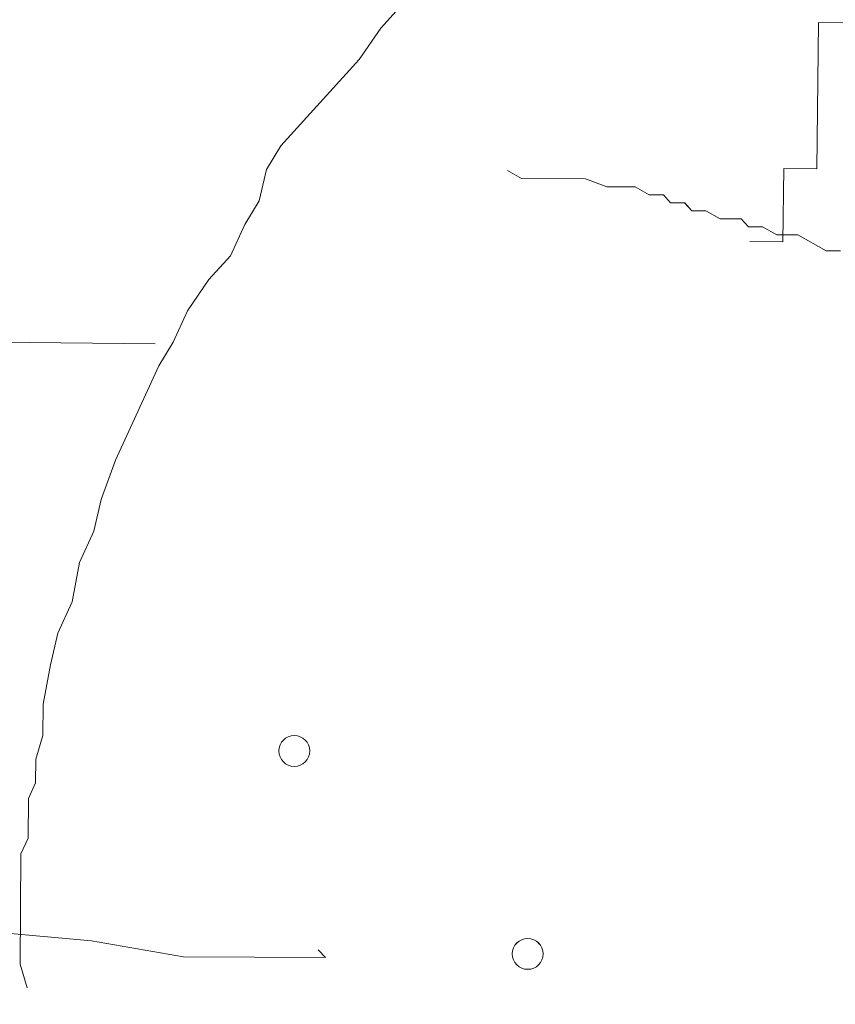
# Model space of a CAD drawing. Units: inches. Extents: x -466983 to 1020, y 324 to 318697.
# Tile 58 of 97: x 640.764 to 643.839, y 938.98 to 942.694. Entities that reach past the tile are written whole.
import ezdxf

# ---------------------------------------------------------------- set-up
doc = ezdxf.new("R2010")
doc.units = ezdxf.units.IN
doc.header["$MEASUREMENT"] = 0
doc.layers.add('A-FLOR-PATT', color=252, linetype='Continuous', lineweight=13)
doc.layers.add('A-FURN', color=8, linetype='Continuous', lineweight=18)

# ---------------------------------------------------------------- blocks, each defined once
blk = doc.blocks.new('L Shaped Sofa')
at = {"ltscale": 2}
for p, q in [((2424.2605, 750.2376), (2424.2127, 750.4005)), ((2424.2558, 749.4786), (2424.2605, 750.2376)), ((2422.162, 750.1932), (2423.1379, 750.1886)), ((2422.2104, 750.1388), (2422.162, 750.1932)), ((2423.1379, 750.1886), (2423.7715, 750.0772)), ((2423.7715, 750.0772), (2424.4056, 750.02)), ((2424.2064, 749.3704), (2424.2558, 749.4786)), ((2424.2047, 749.0993), (2424.2064, 749.3704)), ((2424.1553, 748.9911), (2424.2047, 749.0993)), ((2424.1543, 748.8284), (2424.1553, 748.9911)), ((2424.1045, 748.666), (2424.1543, 748.8284)), ((2424.1032, 748.4492), (2424.1045, 748.666)), ((2424.0527, 748.1783), (2424.1032, 748.4492)), ((2424.0026, 747.9617), (2424.0527, 748.1783)), ((2423.9037, 747.7453), (2424.0026, 747.9617)), ((2423.8532, 747.4744), (2423.9037, 747.7453)), ((2423.7543, 747.258), (2423.8532, 747.4744)), ((2423.7042, 747.0414), (2423.7543, 747.258)), ((2423.6049, 746.7708), (2423.7042, 747.0414)), ((2423.3082, 746.1215), (2423.6049, 746.7708)), ((2423.2096, 745.9594), (2423.3082, 746.1215)), ((2423.1107, 745.7429), (2423.2096, 745.9594)), ((2423.3337, 745.9707), (2428.5509, 745.907)), ((2422.9629, 745.5268), (2423.1107, 745.7429)), ((2422.8156, 745.3648), (2422.9629, 745.5268)), ((2418.6188, 745.3303), (2418.7164, 745.3298)), ((2418.7164, 745.3298), (2418.911, 745.2205)), ((2422.7166, 745.1484), (2422.8156, 745.3648)), ((2419.0084, 744.7638), (2419.0145, 745.2677)), ((2419.0145, 745.2677), (2419.2414, 745.2649)), ((2418.911, 745.2205), (2419.0573, 745.2198)), ((2419.0573, 745.2198), (2419.1546, 745.1651)), ((2419.1546, 745.1651), (2419.2522, 745.1647)), ((2419.2522, 745.1647), (2419.3007, 745.1102)), ((2422.6181, 744.9862), (2422.7166, 745.1484)), ((2419.3007, 745.1102), (2419.447, 745.1095)), ((2419.447, 745.1095), (2419.5443, 745.0549)), ((2419.5443, 745.0549), (2419.6419, 745.0544)), ((2419.6419, 745.0544), (2419.6903, 745)), ((2419.6903, 745), (2419.7879, 744.9995)), ((2419.7879, 744.9995), (2419.8364, 744.9451)), ((2422.5679, 744.7696), (2422.6181, 744.9862)), ((2419.8364, 744.9451), (2419.934, 744.9446)), ((2419.934, 744.9446), (2420.0313, 744.8899)), ((2420.0313, 744.8899), (2420.2264, 744.889)), ((2420.2264, 744.889), (2420.3725, 744.8341)), ((2420.3725, 744.8341), (2420.8116, 744.832)), ((2420.8116, 744.832), (2420.9089, 744.7774)), ((2418.7692, 743.759), (2418.7815, 744.7666)), ((2418.7815, 744.7666), (2419.0084, 744.7638)), ((2422.4693, 744.6074), (2422.5679, 744.7696)), ((2421.9289, 744.0135), (2422.4693, 744.6074)), ((2421.7812, 743.7974), (2421.9289, 744.0135)), ((2421.6339, 743.6354), (2421.7812, 743.7974)), ((2418.5424, 743.7617), (2418.7692, 743.759))]:
    blk.add_line(p, q, dxfattribs=at)
for centre, start, end in [((2420.7699, 750.1679), 90, 270), ((2420.7699, 750.1679), 270, 90), ((2422.3759, 748.7712), 90, 270), ((2422.3759, 748.7712), 270, 90)]:
    blk.add_arc(centre, 0.1062, start, end, dxfattribs=at)

msp = doc.modelspace()

# ---------------------------------------------------------------- hatches: boundary and pattern name
at = {"layer": 'A-FLOR-PATT', "transparency": 33554572}
h = msp.add_hatch(dxfattribs=at)
h.set_pattern_fill('ANSI37', color=256, scale=30)
h.set_pattern_definition([(45, (-1212.4137, -290.035), (-2.6516504, 2.6516504), []), (135, (-1212.4137, -290.035), (-2.6516504, -2.6516504), [])])
h.paths.add_polyline_path([(901.8057, 1075.9377), (900.6144, 1075.9377), (900.6144, 1065.3856), (899.391, 1065.3856), (898.0911, 1065.3856), (892.8356, 1058.7098, -0.258377), (892.1875, 1058.3509), (879.9848, 1058.3509, -0.20177), (879.4382, 1058.5808), (874.0812, 1065.3856), (872.7813, 1065.3856), (871.5579, 1065.3856), (871.5579, 1075.9377), (813.8057, 1075.9377), (813.8057, 1044.7922), (832.3947, 1044.7922, -0.394795), (848.6602, 1028.5356), (848.6602, 1009.9377), (901.8057, 1009.9377), (901.8057, 1015.9377), (901.3057, 1015.9377), (871.3057, 1015.9377), (871.3057, 1017.2502), (871.3344, 1017.2502, -0.401453), (901.3057, 1045.9377), (901.8057, 1045.9377)])
edge = h.paths.add_edge_path(flags=16)
edge.add_line((847.7731, 1068.9486), (847.7731, 1073.7088))
edge.add_arc((849.2269, 1073.7088), 1.4538, 90, 180, ccw=False)
edge.add_line((849.2269, 1075.1627), (864.4921, 1075.1627))
edge.add_arc((864.4921, 1073.7088), 1.4538, 0, 90, ccw=False)
edge.add_line((865.9459, 1073.7088), (865.9459, 1069.0035))
edge.add_arc((832.6447, 1068.9761), 33.3012, -20.61234, 0.04725, ccw=False)
edge.add_ellipse((856.8595, 1058.48), major_axis=(0, 10.2131), ratio=0.6859192, start_angle=100.00884, end_angle=259.99116, ccw=False)
edge.add_arc((881.0742, 1068.9761), 33.3012, 180.04725, 200.61234, ccw=False)
h.paths.add_polyline_path([(853.1456, 1066.4815), (853.1456, 1066.4534), (853.1463, 1066.4534, 0.433107), (852.9166, 1066.6849), (852.9166, 1066.4534), (853.1456, 1066.4534), (853.1456, 1066.4815), (853.088, 1066.6122, 0.697939), (852.6995, 1066.4534), (852.7003, 1066.4534), (852.7003, 1066.4815), (852.9166, 1067.0012), (852.9166, 1066.6849, -0.396254)], flags=0)
h.paths.add_polyline_path([(861.0187, 1066.4815), (861.0187, 1066.4534), (861.0194, 1066.4534, 0.416404), (860.8024, 1066.6849), (860.8024, 1066.4534), (861.0187, 1066.4534), (861.0187, 1066.4815), (860.9672, 1066.6053, 0.713344), (860.5726, 1066.4534), (860.5734, 1066.4534), (860.5734, 1066.4815), (860.8024, 1067.0012), (860.8024, 1066.6849, -0.379973)], flags=0)
edge = h.paths.add_edge_path(flags=0)
edge.add_spline(control_points=[(861.1298, 1065.7855), (861.4661, 1065.2478), (861.6134, 1065.0161), (861.9833, 1064.3736), (862.1924, 1063.9443), (862.5614, 1063.0391), (862.7212, 1062.5633), (862.9865, 1061.5781), (863.092, 1061.0689), (863.2452, 1060.031), (863.293, 1059.5025), (863.3295, 1058.4409), (863.3181, 1057.9078), (863.2366, 1056.8518), (863.1664, 1056.3289), (862.9695, 1055.308), (862.8427, 1054.8099), (862.5365, 1053.8522), (862.3571, 1053.3927), (861.9514, 1052.5249), (861.7251, 1052.1166), (861.233, 1051.3622), (860.9672, 1051.0162), (860.4048, 1050.3949), (860.1082, 1050.1197), (859.4937, 1049.6461), (859.1758, 1049.4476), (858.5276, 1049.1299), (858.1973, 1049.0107), (857.5315, 1048.8518), (857.1959, 1048.8121), (856.5249, 1048.812), (856.1894, 1048.8515), (855.5236, 1049.0101), (855.1933, 1049.1291), (854.545, 1049.4465), (854.2271, 1049.6449), (853.6124, 1050.1183), (853.3158, 1050.3933), (852.7533, 1051.0143), (852.4874, 1051.3602), (851.9952, 1052.1144), (851.7688, 1052.5225), (851.3629, 1053.3902), (851.1834, 1053.8496), (850.877, 1054.8071), (850.7501, 1055.3051), (850.553, 1056.326), (850.4827, 1056.8488), (850.401, 1057.9048), (850.3895, 1058.4379), (850.4257, 1059.4995), (850.4734, 1060.0281), (850.6265, 1061.066), (850.7318, 1061.5753), (850.9969, 1062.5605), (851.1567, 1063.0365), (851.5254, 1063.9418), (851.7345, 1064.3712), (852.1056, 1065.0164), (852.2544, 1065.2503), (852.6082, 1065.7335)], knot_values=[3.915332, 3.915332, 3.915332, 3.915332, 4.013468, 4.013468, 4.175532, 4.175532, 4.337596, 4.337596, 4.49966, 4.49966, 4.661724, 4.661724, 4.823788, 4.823788, 4.985852, 4.985852, 5.147916, 5.147916, 5.30998, 5.30998, 5.472044, 5.472044, 5.634109, 5.634109, 5.796173, 5.796173, 5.958237, 5.958237, 6.120301, 6.120301, 6.282365, 6.282365, 6.444429, 6.444429, 6.606493, 6.606493, 6.768557, 6.768557, 6.930621, 6.930621, 7.092685, 7.092685, 7.254749, 7.254749, 7.416813, 7.416813, 7.578878, 7.578878, 7.740942, 7.740942, 7.903006, 7.903006, 8.06507, 8.06507, 8.227134, 8.227134, 8.389198, 8.389198, 8.551262, 8.551262, 8.65037, 8.65037, 8.65037, 8.65037], degree=3, periodic=0)
edge.add_line((852.6421, 1065.7855), (861.1298, 1065.7855))
edge = h.paths.add_edge_path(flags=0)
edge.add_ellipse((856.8496, 1057.7432), major_axis=(0, 7.7921), ratio=0.687861, start_angle=0, end_angle=360)
h.paths.add_polyline_path([(848.8634, 1069.3891), (848.8634, 1073.9605, -0.414214), (849.9538, 1075.0508), (863.7652, 1075.0508, -0.414214), (864.8555, 1073.9605), (864.8555, 1069.3891, -0.388936), (864.5237, 1069.027, -0.043561), (849.1953, 1069.027, -0.388936)], flags=0)
h.paths.add_polyline_path([(853.1006, 1068.1122, -1), (852.6775, 1068.1122, -1)], flags=0)
edge = h.paths.add_edge_path(flags=0)
edge.add_ellipse((856.8595, 1057.3378), major_axis=(0, 2.207), ratio=0.657164, start_angle=0, end_angle=360)
h.paths.add_polyline_path([(861.0415, 1068.1122, -1), (860.6184, 1068.1122, -1)], flags=0)
edge = h.paths.add_edge_path()
edge.add_line((573.9537, 1057.3412), (573.9537, 1075.9377))
edge.add_line((573.9537, 1075.9377), (558.7308, 1075.9377))
edge.add_line((558.7308, 1075.9377), (558.7308, 1065.3856))
edge.add_line((558.7308, 1065.3856), (557.5074, 1065.3856))
edge.add_line((557.5074, 1065.3856), (556.2075, 1065.3856))
edge.add_line((556.2075, 1065.3856), (550.952, 1058.7098))
edge.add_arc((550.3039, 1059.1155), 0.7646, 270, 327.9483, ccw=False)
edge.add_line((550.3039, 1058.3509), (538.1012, 1058.3509))
edge.add_arc((538.1012, 1059.1155), 0.7646, 224.3704, 270, ccw=False)
edge.add_line((537.5546, 1058.5808), (532.1976, 1065.3856))
edge.add_line((532.1976, 1065.3856), (530.8977, 1065.3856))
edge.add_line((530.8977, 1065.3856), (529.6743, 1065.3856))
edge.add_line((529.6743, 1065.3856), (529.6743, 1075.9377))
edge.add_line((529.6743, 1075.9377), (520.8057, 1075.9377))
edge.add_line((520.8057, 1075.9377), (520.8057, 1045.9377))
edge.add_line((520.8057, 1045.9377), (521.3057, 1045.9377))
edge.add_arc((521.3057, 1015.9377), 30, 2.50749, 90, ccw=False)
edge.add_line((551.277, 1017.2502), (551.3057, 1017.2502))
edge.add_line((551.3057, 1017.2502), (551.3057, 1015.9377))
edge.add_line((551.3057, 1015.9377), (520.8057, 1015.9377))
edge.add_line((520.8057, 1015.9377), (520.8057, 1009.9377))
edge.add_line((520.8057, 1009.9377), (559.1913, 1010.4022))
edge.add_arc((559.1913, 1011.856), 1.4538, 180, 270, ccw=False)
edge.add_line((557.7375, 1011.856), (557.7375, 1016.5613))
edge.add_arc((591.0386, 1016.5888), 33.3012, 159.38766, 180.04725, ccw=False)
edge.add_ellipse((566.8239, 1027.0848), major_axis=(0, 10.2131), ratio=0.6859192, start_angle=280.00884, end_angle=439.99116, ccw=False)
edge.add_arc((542.6091, 1016.5888), 33.3012, 0.04725, 20.61234, ccw=False)
edge.add_line((575.9103, 1016.6162), (575.9103, 1011.856))
edge.add_arc((574.4565, 1011.856), 1.4538, -90, 0, ccw=False)
edge.add_line((574.4565, 1010.4022), (608.8057, 1009.9377))
edge.add_line((608.8057, 1009.9377), (608.8057, 1041.0857))
edge.add_line((608.8057, 1041.0857), (590.2179, 1041.0857))
edge.add_arc((590.775, 1057.9074), 16.8309, 181.92775, 268.10321, ccw=False)
edge = h.paths.add_edge_path()
edge.add_ellipse((494.2443, 583.6204), major_axis=(0, 10.2131), ratio=0.6859192, start_angle=280.00884, end_angle=439.99116, ccw=False)
edge.add_arc((470.0296, 573.1243), 33.3012, 0.04725, 20.61234, ccw=False)
edge.add_line((503.3307, 573.1518), (503.3307, 568.3916))
edge.add_arc((501.8769, 568.3916), 1.4538, -90, 0, ccw=False)
edge.add_line((501.8769, 566.9377), (539.8057, 566.9377))
edge.add_line((539.8057, 566.9377), (539.8057, 572.9377))
edge.add_line((539.8057, 572.9377), (539.3057, 572.9377))
edge.add_line((539.3057, 572.9377), (509.3057, 572.9377))
edge.add_line((509.3057, 572.9377), (509.3057, 574.2502))
edge.add_line((509.3057, 574.2502), (509.3344, 574.2502))
edge.add_arc((539.3057, 572.9377), 30, 90, 177.49251, ccw=False)
edge.add_line((539.3057, 602.9377), (539.8057, 602.9377))
edge.add_line((539.8057, 602.9377), (539.8057, 626.9377))
edge.add_line((539.8057, 626.9377), (531.7718, 626.9377))
edge.add_line((531.7718, 626.9377), (531.7718, 616.3856))
edge.add_line((531.7718, 616.3856), (530.5484, 616.3856))
edge.add_line((530.5484, 616.3856), (529.2485, 616.3856))
edge.add_line((529.2485, 616.3856), (523.7105, 609.3509))
edge.add_line((523.7105, 609.3509), (510.7766, 609.3509))
edge.add_line((510.7766, 609.3509), (505.2386, 616.3856))
edge.add_line((505.2386, 616.3856), (503.9387, 616.3856))
edge.add_line((503.9387, 616.3856), (502.7153, 616.3856))
edge.add_line((502.7153, 616.3856), (502.7153, 626.9377))
edge.add_line((502.7153, 626.9377), (481.6983, 626.9377))
edge.add_line((481.6983, 626.9377), (481.6983, 610.995))
edge.add_arc((467.2703, 611.4728), 14.4359, 271.92775, 358.10321, ccw=False)
edge.add_line((467.7559, 597.0451), (451.8057, 597.0451))
edge.add_line((451.8057, 597.0451), (451.8057, 584.4035))
edge.add_line((451.8057, 584.4035), (451.8057, 566.9377))
edge.add_line((451.8057, 566.9377), (486.6117, 566.9377))
edge.add_arc((486.6117, 568.3916), 1.4538, 180, 270, ccw=False)
edge.add_line((485.1579, 568.3916), (485.1579, 573.0969))
edge.add_arc((518.4591, 573.1243), 33.3012, 159.38766, 180.04725, ccw=False)
h.paths.add_polyline_path([(836.2609, 1020.7328), (879.8898, 1020.7328), (879.8898, 1039.3902), (836.2609, 1039.3902)], flags=25)
h.paths.add_polyline_path([(549.9851, 1036.7492), (593.614, 1036.7492), (593.614, 1055.4065), (549.9851, 1055.4065)], flags=24)
h.paths.add_polyline_path([(475.123, 595.5959), (518.752, 595.5959), (518.752, 614.2532), (475.123, 614.2532)], flags=24)
h = msp.add_hatch(dxfattribs=at)
h.set_pattern_fill('ANSI37', color=256, scale=20)
h.set_pattern_definition([(45, (-1212.4137, -290.035), (-1.767767, 1.767767), []), (135, (-1212.4137, -290.035), (-1.767767, -1.767767), [])])
h.paths.add_polyline_path([(809.8057, 870.9377), (809.8057, 888.1519), (806.9985, 888.1519), (802.6624, 888.1519), (789.3832, 888.1519), (786.2846, 888.1519, -0.414214), (785.4991, 888.9374), (785.4991, 900.1959), (785.4991, 908.4696, -0.414214), (786.8082, 909.7787, -0.414214), (785.4991, 911.0878), (785.4991, 929.1015, -0.414214), (786.8082, 930.4106, -0.414214), (785.4991, 931.7197), (785.4991, 931.9039, -0.414214), (784.19, 930.5948), (766.7223, 930.5948, -0.412359), (765.4132, 931.8956, -0.413741), (764.1145, 930.5782), (744.5781, 930.422, -0.416556), (743.7864, 931.2075), (743.7864, 933.5153), (742.2154, 933.5153), (742.2154, 952.024, -0.001344), (743.7864, 952.1998), (743.7864, 953.9377), (678.5915, 953.9377), (678.5915, 951.1305), (678.5915, 946.7945), (678.5915, 933.5153), (678.5915, 930.4166, -0.414214), (677.806, 929.6312), (666.5475, 929.6312), (658.2738, 929.6312, -0.414214), (656.9647, 930.9403, -0.414214), (655.6556, 929.6312), (637.6419, 929.6312, -0.414214), (636.3328, 930.9403, -0.414214), (635.0237, 929.6312), (634.8395, 929.6312, -0.414214), (636.1486, 928.322), (636.1486, 910.8544, -0.412359), (634.8478, 909.5452, -0.413741), (636.1653, 908.2466), (636.3214, 888.7102, -0.416556), (635.5359, 887.9184), (633.2281, 887.9184), (633.2281, 886.3475), (614.7194, 886.3475, -0.001344), (614.5436, 887.9184), (612.8057, 887.9184), (612.8057, 834.9377), (612.8057, 752.9377), (612.8057, 748.9377), (612.8057, 697.9377), (654.8057, 697.9377), (654.8057, 701.9377), (715.8057, 701.9377), (715.8057, 737.4353), (774.2918, 737.4353), (774.2918, 795.9377), (809.8057, 795.9377)])
h.paths.add_polyline_path([(679.2761, 849.5757, 0.102523), (682.1475, 849.2608, -0.080461), (694.5428, 849.7725, -0.283899), (694.4822, 849.0082, 0.136605), (694.4068, 848.8103, -0.030441), (694.5428, 846.8929), (694.5428, 842.6198), (694.5428, 838.3466, -0.028219), (694.4246, 836.5684), (694.425, 836.5684, 0.196187), (694.4456, 836.2708, -0.302897), (694.5428, 835.467, -0.080461), (682.1475, 835.9787, 0.102523), (679.2761, 835.6638, -0.58611), (678.6457, 836.0169), (678.6457, 849.2227, -0.58611)], flags=16)
h.paths.add_polyline_path([(679.5173, 848.6515, 0.699597), (679.476, 848.6342, 1.20716), (679.1935, 848.7422, 0.010621)], flags=0)
h.paths.add_polyline_path([(679.4923, 836.5608, -0.013798), (679.9178, 836.6594, -0.071703), (682.8533, 837.1434, -0.165743), (682.1665, 839.1006), (682.1665, 842.6094), (682.1665, 846.0603, -0.240616), (683.4733, 848.6767, -0.068263), (693.9295, 849.0082), (693.7875, 848.7083), (693.7875, 849.0228, 0.067332), (683.4733, 848.6767, 0.240616), (682.1665, 846.0603), (682.1665, 842.6094), (682.1665, 839.1006, 0.23459), (683.461, 836.5513, 0.068093), (693.7875, 836.1955), (693.7875, 836.5104), (693.9296, 836.2102, -0.077215), (682.2421, 836.7815, 0.086627), (679.5283, 836.5701, -0.628402), (679.5029, 836.5735), (679.5029, 836.6071, 0.910458)], flags=0)
h.paths.add_polyline_path([(679.476, 848.6364), (679.2069, 848.647), (679.2069, 836.5718, 0.913566), (679.3645, 836.5861), (679.476, 836.5824)], flags=0)
h.paths.add_polyline_path([(679.2761, 829.8604, 0.102523), (682.1475, 829.5455, -0.080461), (694.5428, 830.0572, -0.283899), (694.4822, 829.2929, 0.136605), (694.4068, 829.095, -0.030441), (694.5428, 827.1776), (694.5428, 822.9045), (694.5428, 818.6314, -0.028219), (694.4246, 816.8531), (694.425, 816.8532, 0.196187), (694.4456, 816.5555, -0.302897), (694.5428, 815.7517, -0.080461), (682.1475, 816.2635, 0.102523), (679.2761, 815.9485, -0.58611), (678.6457, 816.3016), (678.6457, 829.5074, -0.58611)], flags=16)
h.paths.add_polyline_path([(679.5173, 828.9362, 0.699597), (679.476, 828.9189, 1.20716), (679.1935, 829.0269, 0.010621)], flags=0)
h.paths.add_polyline_path([(679.4923, 816.8456, -0.013798), (679.9178, 816.9441, -0.071703), (682.8533, 817.4281, -0.165743), (682.1665, 819.3853), (682.1665, 822.8941), (682.1665, 826.345, -0.240616), (683.4733, 828.9614, -0.068263), (693.9295, 829.2929), (693.7875, 828.9931), (693.7875, 829.3076, 0.067332), (683.4733, 828.9614, 0.240616), (682.1665, 826.345), (682.1665, 822.8941), (682.1665, 819.3853, 0.23459), (683.461, 816.836, 0.068093), (693.7875, 816.4802), (693.7875, 816.7952), (693.9296, 816.4949, -0.077215), (682.2421, 817.0662, 0.086627), (679.5283, 816.8549, -0.628402), (679.5029, 816.8582), (679.5029, 816.8918, 0.910458)], flags=0)
h.paths.add_polyline_path([(679.476, 828.9211), (679.2069, 828.9317), (679.2069, 816.8565, 0.913566), (679.3645, 816.8708), (679.476, 816.8671)], flags=0)
h.paths.add_polyline_path([(679.2761, 810.1451, 0.102523), (682.1475, 809.8302, -0.080461), (694.5428, 810.342, -0.3023), (694.4466, 809.5394, 0.10023), (694.4058, 809.3878, -0.03057), (694.5428, 807.4623), (694.5428, 803.1892), (694.5428, 798.9161, -0.03057), (694.4058, 796.9906, 0.10023), (694.4466, 796.839, -0.3023), (694.5428, 796.0365, -0.080461), (682.1475, 796.5482, 0.102523), (679.2761, 796.2333, -0.58611), (678.6457, 796.5863), (678.6457, 809.7921, -0.58611)], flags=16)
h.paths.add_polyline_path([(679.5173, 809.2417, 0.699597), (679.476, 809.2244, 1.20716), (679.1935, 809.3324, 0.010621)], flags=0)
h.paths.add_polyline_path([(679.4923, 797.151, -0.013798), (679.9178, 797.2496, -0.071703), (682.8533, 797.7336, -0.165743), (682.1665, 799.6908), (682.1665, 803.1996), (682.1665, 806.6505, -0.239349), (683.461, 809.2577, -0.072465), (694.4468, 809.5405, 0.197932), (694.425, 809.2405), (693.7875, 809.2985), (693.7875, 809.6135, 0.068093), (683.461, 809.2577, 0.239349), (682.1665, 806.6505), (682.1665, 803.1996), (682.1665, 799.6908, 0.235854), (683.4733, 797.1323, 0.067332), (693.7875, 796.7861), (693.7875, 797.1006), (694.425, 797.1586, 0.197932), (694.4468, 796.8586, -0.080419), (682.1557, 797.3795, 0.083867), (679.5283, 797.1603, -0.628402), (679.5029, 797.1637), (679.5029, 797.1973, 0.910458)], flags=0)
h.paths.add_polyline_path([(679.2069, 809.2372), (679.2069, 797.162, 0.913566), (679.3645, 797.1763), (679.476, 797.1726), (679.476, 809.2266)], flags=0)
h.paths.add_polyline_path([(695.3643, 853.2989), (728.2231, 853.2989), (728.2231, 771.1519), (695.3643, 771.1519)], flags=16)
h.paths.add_polyline_path([(696.0215, 852.6417), (727.5659, 852.6417), (727.5659, 771.809), (696.0215, 771.809)], flags=0)
h.paths.add_polyline_path([(679.2761, 788.7869, 0.102523), (682.1475, 788.472, -0.080461), (694.5428, 788.9837, -0.3023), (694.4466, 788.1812, 0.10023), (694.4058, 788.0296, -0.03057), (694.5428, 786.1041), (694.5428, 781.831), (694.5428, 777.5578, -0.03057), (694.4058, 775.6323, 0.10023), (694.4466, 775.4808, -0.3023), (694.5428, 774.6782, -0.080461), (682.1475, 775.19, 0.102523), (679.2761, 774.875, -0.58611), (678.6457, 775.2281), (678.6457, 788.4339, -0.58611)], flags=16)
h.paths.add_polyline_path([(679.5173, 787.8834, 0.699597), (679.476, 787.8662, 1.20716), (679.1935, 787.9742, 0.010621)], flags=0)
h.paths.add_polyline_path([(679.4923, 775.7928, -0.013798), (679.9178, 775.8914, -0.071703), (682.8533, 776.3753, -0.165743), (682.1665, 778.3325), (682.1665, 781.8414), (682.1665, 785.2922, -0.239349), (683.461, 787.8995, -0.072465), (694.4468, 788.1823, 0.197932), (694.425, 787.8823), (693.7875, 787.9403), (693.7875, 788.2553, 0.068093), (683.461, 787.8995, 0.239349), (682.1665, 785.2922), (682.1665, 781.8414), (682.1665, 778.3325, 0.235854), (683.4733, 775.7741, 0.067332), (693.7875, 775.4279), (693.7875, 775.7424), (694.425, 775.8004, 0.197932), (694.4468, 775.5004, -0.080419), (682.1557, 776.0212, 0.083867), (679.5283, 775.8021, -0.628402), (679.5029, 775.8054), (679.5029, 775.8391, 0.910458)], flags=0)
h.paths.add_polyline_path([(679.2069, 787.8789), (679.2069, 775.8038, 0.913566), (679.3645, 775.818), (679.476, 775.8144), (679.476, 787.8684)], flags=0)
h.paths.add_polyline_path([(704.641, 854.1204, -0.080461), (705.1527, 866.5157, 0.102523), (704.8378, 869.3871, -0.58611), (705.1908, 870.0174), (718.3966, 870.0174, -0.58611), (718.7496, 869.3871, 0.102523), (718.4347, 866.5157, -0.080461), (718.9465, 854.1204, -0.3023), (718.1439, 854.2166, 0.10023), (717.9924, 854.2574, -0.03057), (716.0668, 854.1204), (711.7937, 854.1204), (707.5206, 854.1204, -0.03057), (705.5951, 854.2574, 0.10023), (705.4435, 854.2166, -0.3023)], flags=16)
h.paths.add_polyline_path([(717.8462, 869.1459, 0.699597), (717.8289, 869.1872, 1.20716), (717.9369, 869.4697, 0.010621)], flags=0)
h.paths.add_polyline_path([(705.4631, 854.2164, -0.080419), (705.984, 866.5074, 0.083867), (705.7648, 869.1349, -0.628402), (705.7682, 869.1603), (705.8018, 869.1603, 0.910458), (705.7555, 869.1709, -0.013798), (705.8541, 868.7454, -0.071703), (706.3381, 865.8099, -0.165743), (708.2953, 866.4967), (711.8041, 866.4967), (715.255, 866.4967, -0.239349), (717.8622, 865.2022, -0.072465), (718.145, 854.2164, 0.197932), (717.845, 854.2382), (717.903, 854.8757), (718.218, 854.8757, 0.068093), (717.8622, 865.2022, 0.239349), (715.255, 866.4967), (711.8041, 866.4967), (708.2953, 866.4967, 0.235854), (705.7368, 865.1898, 0.067332), (705.3906, 854.8757), (705.7051, 854.8757), (705.7631, 854.2382, 0.197932)], flags=16)
h.paths.add_polyline_path([(705.7665, 869.4563, 0.913566), (705.7808, 869.2987), (705.7771, 869.1872), (717.8311, 869.1872), (717.8417, 869.4563)], flags=0)
h.paths.add_polyline_path([(729.0446, 842.6198), (729.0446, 846.8929, -0.03057), (729.1817, 848.8184, 0.10023), (729.1408, 848.9699, -0.3023), (729.0446, 849.7725, -0.080461), (741.4399, 849.2608, 0.102523), (744.3113, 849.5757, -0.58611), (744.9417, 849.2227), (744.9417, 836.0169, -0.58611), (744.3113, 835.6638, 0.102523), (741.4399, 835.9787, -0.080461), (729.0446, 835.467, -0.3023), (729.1408, 836.2696, 0.10023), (729.1817, 836.4211, -0.03057), (729.0446, 838.3466)], flags=16)
h.paths.add_polyline_path([(744.1115, 836.5846, 1.20716), (744.3939, 836.4766, 0.010621), (744.0701, 836.5673, 0.699597)], flags=0)
h.paths.add_polyline_path([(729.1407, 836.2684, 0.197932), (729.1624, 836.5684), (729.7999, 836.5104), (729.7999, 836.1955, 0.068093), (740.1264, 836.5513, 0.239349), (741.4209, 839.1585), (741.4209, 842.6094), (741.4209, 846.1182, 0.235854), (740.1141, 848.6767, 0.067332), (729.7999, 849.0228), (729.7999, 848.7083), (729.1624, 848.6503, 0.197932), (729.1407, 848.9504, -0.080419), (741.4317, 848.4295, 0.083867), (744.0591, 848.6486, -0.628402), (744.0845, 848.6453), (744.0845, 848.6117, 0.910458), (744.0951, 848.6579, -0.013798), (743.6696, 848.5594, -0.071703), (740.7341, 848.0754, -0.165743), (741.4209, 846.1182), (741.4209, 842.6094), (741.4209, 839.1585, -0.239349), (740.1264, 836.5513, -0.072465)], flags=0)
h.paths.add_polyline_path([(729.0446, 830.0572, -0.080461), (741.4399, 829.5455, 0.102523), (744.3113, 829.8604, -0.58611), (744.9417, 829.5074), (744.9417, 816.3016, -0.58611), (744.3113, 815.9485, 0.102523), (741.4399, 816.2635, -0.080461), (729.0446, 815.7517, -0.3023), (729.1408, 816.5543, 0.10023), (729.1817, 816.7058, -0.03057), (729.0446, 818.6314), (729.0446, 822.9045), (729.0446, 827.1776, -0.03057), (729.1817, 829.1031, 0.10023), (729.1408, 829.2547, -0.3023)], flags=16)
h.paths.add_polyline_path([(744.1115, 816.8693, 1.20716), (744.3939, 816.7613, 0.010621), (744.0701, 816.852, 0.699597)], flags=0)
h.paths.add_polyline_path([(729.1407, 829.2351, -0.080419), (741.4317, 828.7142, 0.083867), (744.0591, 828.9334, -0.628402), (744.0845, 828.93), (744.0845, 828.8964, 0.910458), (744.0951, 828.9427, -0.013798), (743.6696, 828.8441, -0.071703), (740.7341, 828.3601, -0.165743), (741.4209, 826.4029), (741.4209, 822.8941), (741.4209, 819.4432, -0.239349), (740.1264, 816.836, -0.072465), (729.1407, 816.5531, 0.197932), (729.1624, 816.8532), (729.7999, 816.7952), (729.7999, 816.4802, 0.068093), (740.1264, 816.836, 0.239349), (741.4209, 819.4432), (741.4209, 822.8941), (741.4209, 826.4029, 0.235854), (740.1141, 828.9614, 0.067332), (729.7999, 829.3076), (729.7999, 828.9931), (729.1624, 828.9351, 0.197932)], flags=16)
h.paths.add_polyline_path([(729.0446, 810.342, -0.080461), (741.4399, 809.8302, 0.102523), (744.3113, 810.1451, -0.58611), (744.9417, 809.7921), (744.9417, 796.5863, -0.58611), (744.3113, 796.2333, 0.102523), (741.4399, 796.5482, -0.080461), (729.0446, 796.0365, -0.283899), (729.1052, 796.8007, 0.136605), (729.1806, 796.9987, -0.030441), (729.0446, 798.9161), (729.0446, 803.1892), (729.0446, 807.4623, -0.028219), (729.1628, 809.2406), (729.1624, 809.2405, 0.196187), (729.1418, 809.5382, -0.302897)], flags=16)
h.paths.add_polyline_path([(744.1115, 797.1748, 1.20716), (744.3939, 797.0668, 0.010621), (744.0701, 797.1575, 0.699597)], flags=0)
h.paths.add_polyline_path([(741.3453, 809.0275, 0.086627), (744.0591, 809.2388, -0.628402), (744.0845, 809.2355), (744.0845, 809.2019, 0.910458), (744.0951, 809.2481, -0.013798), (743.6696, 809.1496, -0.071703), (740.7341, 808.6656, -0.165743), (741.4209, 806.7084), (741.4209, 803.1996), (741.4209, 799.7487, -0.240616), (740.1141, 797.1323, -0.068263), (729.658, 796.8008), (729.7999, 797.1006), (729.7999, 796.7861, 0.067332), (740.1141, 797.1323, 0.240616), (741.4209, 799.7487), (741.4209, 803.1996), (741.4209, 806.7084, 0.23459), (740.1264, 809.2577, 0.068093), (729.7999, 809.6135), (729.7999, 809.2985), (729.6578, 809.5988, -0.077215)], flags=0)
h.paths.add_polyline_path([(704.641, 770.3304, -0.283899), (705.4053, 770.2697, 0.136605), (705.6032, 770.1944, -0.030441), (707.5206, 770.3304), (711.7937, 770.3304), (716.0668, 770.3304, -0.028219), (717.8451, 770.2122), (717.845, 770.2126, 0.196187), (718.1427, 770.2331, -0.302897), (718.9465, 770.3304, -0.080461), (718.4347, 757.9351, 0.102523), (718.7496, 755.0637, -0.58611), (718.3966, 754.4333), (705.1908, 754.4333, -0.58611), (704.8378, 755.0637, 0.102523), (705.1527, 757.9351, -0.080461)], flags=16)
h.paths.add_polyline_path([(705.762, 755.3048, 0.699597), (705.7793, 755.2635, 1.20716), (705.6713, 754.9811, 0.010621)], flags=0)
h.paths.add_polyline_path([(705.4053, 769.717), (705.7051, 769.5751), (705.3906, 769.5751, 0.067332), (705.7368, 759.2609, 0.240616), (708.3532, 757.954), (711.8041, 757.954), (715.3129, 757.954, 0.23459), (717.8622, 759.2485, 0.068093), (718.218, 769.5751), (717.903, 769.5751), (718.2033, 769.7172, -0.077215), (717.632, 758.0297, 0.086627), (717.8433, 755.3159, -0.628402), (717.84, 755.2904), (717.8064, 755.2904, 0.910458), (717.8526, 755.2799, -0.013798), (717.7541, 755.7053, -0.071703), (717.2701, 758.6409, -0.165743), (715.3129, 757.954), (711.8041, 757.954), (708.3532, 757.954, -0.240616), (705.7368, 759.2609, -0.068263)], flags=0)
h.paths.add_polyline_path([(729.0446, 788.9837, -0.080461), (741.4399, 788.472, 0.102523), (744.3113, 788.7869, -0.58611), (744.9417, 788.4339), (744.9417, 775.2281, -0.58611), (744.3113, 774.875, 0.102523), (741.4399, 775.19, -0.080461), (729.0446, 774.6782, -0.283899), (729.1052, 775.4425, 0.136605), (729.1806, 775.6405, -0.030441), (729.0446, 777.5578), (729.0446, 781.831), (729.0446, 786.1041, -0.028219), (729.1628, 787.8823), (729.1624, 787.8823, 0.196187), (729.1418, 788.1799, -0.302897)], flags=16)
h.paths.add_polyline_path([(744.1115, 775.8165, 1.20716), (744.3939, 775.7086, 0.010621), (744.0701, 775.7993, 0.699597)], flags=0)
h.paths.add_polyline_path([(741.3453, 787.6692, 0.086627), (744.0591, 787.8806, -0.628402), (744.0845, 787.8773), (744.0845, 787.8437, 0.910458), (744.0951, 787.8899, -0.013798), (743.6696, 787.7913, -0.071703), (740.7341, 787.3074, -0.165743), (741.4209, 785.3502), (741.4209, 781.8414), (741.4209, 778.3905, -0.240616), (740.1141, 775.7741, -0.068263), (729.658, 775.4425), (729.7999, 775.7424), (729.7999, 775.4279, 0.067332), (740.1141, 775.7741, 0.240616), (741.4209, 778.3905), (741.4209, 781.8414), (741.4209, 785.3502, 0.23459), (740.1264, 787.8995, 0.068093), (729.7999, 788.2553), (729.7999, 787.9403), (729.6578, 788.2405, -0.077215)], flags=0)
h.paths.add_polyline_path([(744.1115, 848.6364), (744.1115, 836.5824), (744.3805, 836.5718), (744.3805, 848.647, 0.913566), (744.2229, 848.6327)], flags=0)
h.paths.add_polyline_path([(744.2229, 828.9174), (744.1115, 828.9211), (744.1115, 816.8671), (744.3805, 816.8565), (744.3805, 828.9317, 0.913566)], flags=0)
h.paths.add_polyline_path([(717.8311, 755.2635), (705.7771, 755.2635), (705.7665, 754.9945), (717.8417, 754.9945, 0.913566), (717.8274, 755.1521)], flags=0)
h.paths.add_polyline_path([(744.2229, 809.2229), (744.1115, 809.2266), (744.1115, 797.1726), (744.3805, 797.162), (744.3805, 809.2372, 0.913566)], flags=0)
h.paths.add_polyline_path([(744.1115, 787.8684), (744.1115, 775.8144), (744.3805, 775.8038), (744.3805, 787.8789, 0.913566), (744.2229, 787.8647)], flags=0)
h.paths.add_polyline_path([(678.8774, 877.1228), (737.6127, 877.1228), (737.6127, 899.5116), (678.8774, 899.5116)], flags=24)

# ---------------------------------------------------------------- linework, layer by layer
at = {"layer": 'A-FURN', "ltscale": 2}
for p, q in [((642.2059, 942.7509), (642.1251, 942.6621)), ((642.2059, 942.7509), (642.1251, 942.6621)), ((642.2059, 942.7509), (642.1251, 942.6621)), ((642.2059, 942.7509), (642.1251, 942.6621)), ((642.2059, 942.7509), (642.1251, 942.6621)), ((642.2059, 942.7509), (642.1251, 942.6621)), ((642.1251, 942.6621), (642.0441, 942.5436)), ((642.1251, 942.6621), (642.0441, 942.5436)), ((642.1251, 942.6621), (642.0441, 942.5436)), ((642.1251, 942.6621), (642.0441, 942.5436)), ((642.1251, 942.6621), (642.0441, 942.5436)), ((642.1251, 942.6621), (642.0441, 942.5436)), ((643.7763, 942.6831), (643.7696, 942.1307)), ((643.7763, 942.6831), (643.7696, 942.1307)), ((643.7763, 942.6831), (643.7696, 942.1307)), ((643.7763, 942.6831), (643.7696, 942.1307)), ((643.7763, 942.6831), (643.7696, 942.1307)), ((643.7763, 942.6831), (643.7696, 942.1307)), ((643.9007, 942.6816), (643.7763, 942.6831)), ((643.9007, 942.6816), (643.7763, 942.6831)), ((643.9007, 942.6816), (643.7763, 942.6831)), ((643.9007, 942.6816), (643.7763, 942.6831)), ((643.9007, 942.6816), (643.7763, 942.6831)), ((643.9007, 942.6816), (643.7763, 942.6831)), ((642.0441, 942.5436), (641.7479, 942.218)), ((642.0441, 942.5436), (641.7479, 942.218)), ((642.0441, 942.5436), (641.7479, 942.218)), ((642.0441, 942.5436), (641.7479, 942.218)), ((642.0441, 942.5436), (641.7479, 942.218)), ((642.0441, 942.5436), (641.7479, 942.218)), ((641.7479, 942.218), (641.6938, 942.1291)), ((641.7479, 942.218), (641.6938, 942.1291)), ((641.7479, 942.218), (641.6938, 942.1291)), ((641.7479, 942.218), (641.6938, 942.1291)), ((641.7479, 942.218), (641.6938, 942.1291)), ((641.7479, 942.218), (641.6938, 942.1291)), ((641.6938, 942.1291), (641.6663, 942.0103)), ((641.6938, 942.1291), (641.6663, 942.0103)), ((641.6938, 942.1291), (641.6663, 942.0103)), ((641.6938, 942.1291), (641.6663, 942.0103)), ((641.6938, 942.1291), (641.6663, 942.0103)), ((641.6938, 942.1291), (641.6663, 942.0103)), ((642.6566, 942.0948), (642.6033, 942.1248)), ((642.6566, 942.0948), (642.6033, 942.1248)), ((642.6566, 942.0948), (642.6033, 942.1248)), ((642.6566, 942.0948), (642.6033, 942.1248)), ((642.6566, 942.0948), (642.6033, 942.1248)), ((642.6566, 942.0948), (642.6033, 942.1248)), ((643.6452, 942.1322), (643.6418, 941.856)), ((643.6452, 942.1322), (643.6418, 941.856)), ((643.6452, 942.1322), (643.6418, 941.856)), ((643.6452, 942.1322), (643.6418, 941.856)), ((643.6452, 942.1322), (643.6418, 941.856)), ((643.6452, 942.1322), (643.6418, 941.856)), ((643.7696, 942.1307), (643.6452, 942.1322)), ((643.7696, 942.1307), (643.6452, 942.1322)), ((643.7696, 942.1307), (643.6452, 942.1322)), ((643.7696, 942.1307), (643.6452, 942.1322)), ((643.7696, 942.1307), (643.6452, 942.1322)), ((643.7696, 942.1307), (643.6452, 942.1322)), ((642.8974, 942.0937), (642.6566, 942.0948)), ((642.8974, 942.0937), (642.6566, 942.0948)), ((642.8974, 942.0937), (642.6566, 942.0948)), ((642.8974, 942.0937), (642.6566, 942.0948)), ((642.8974, 942.0937), (642.6566, 942.0948)), ((642.8974, 942.0937), (642.6566, 942.0948)), ((642.9775, 942.0636), (642.8974, 942.0937)), ((642.9775, 942.0636), (642.8974, 942.0937)), ((642.9775, 942.0636), (642.8974, 942.0937)), ((642.9775, 942.0636), (642.8974, 942.0937)), ((642.9775, 942.0636), (642.8974, 942.0937)), ((642.9775, 942.0636), (642.8974, 942.0937)), ((643.0845, 942.0631), (642.9775, 942.0636)), ((643.0845, 942.0631), (642.9775, 942.0636)), ((643.0845, 942.0631), (642.9775, 942.0636)), ((643.0845, 942.0631), (642.9775, 942.0636)), ((643.0845, 942.0631), (642.9775, 942.0636)), ((643.0845, 942.0631), (642.9775, 942.0636)), ((643.1378, 942.0331), (643.0845, 942.0631)), ((643.1378, 942.0331), (643.0845, 942.0631)), ((643.1378, 942.0331), (643.0845, 942.0631)), ((643.1378, 942.0331), (643.0845, 942.0631)), ((643.1378, 942.0331), (643.0845, 942.0631)), ((643.1378, 942.0331), (643.0845, 942.0631)), ((643.1913, 942.0329), (643.1378, 942.0331)), ((643.1913, 942.0329), (643.1378, 942.0331)), ((643.1913, 942.0329), (643.1378, 942.0331)), ((643.1913, 942.0329), (643.1378, 942.0331)), ((643.1913, 942.0329), (643.1378, 942.0331)), ((643.1913, 942.0329), (643.1378, 942.0331)), ((643.2179, 942.003), (643.1913, 942.0329)), ((643.2179, 942.003), (643.1913, 942.0329)), ((643.2179, 942.003), (643.1913, 942.0329)), ((643.2179, 942.003), (643.1913, 942.0329)), ((643.2179, 942.003), (643.1913, 942.0329)), ((643.2179, 942.003), (643.1913, 942.0329)), ((641.6663, 942.0103), (641.6123, 941.9214)), ((641.6663, 942.0103), (641.6123, 941.9214)), ((641.6663, 942.0103), (641.6123, 941.9214)), ((641.6663, 942.0103), (641.6123, 941.9214)), ((641.6663, 942.0103), (641.6123, 941.9214)), ((641.6663, 942.0103), (641.6123, 941.9214)), ((643.2714, 942.0028), (643.2179, 942.003)), ((643.2714, 942.0028), (643.2179, 942.003)), ((643.2714, 942.0028), (643.2179, 942.003)), ((643.2714, 942.0028), (643.2179, 942.003)), ((643.2714, 942.0028), (643.2179, 942.003)), ((643.2714, 942.0028), (643.2179, 942.003)), ((643.2979, 941.9729), (643.2714, 942.0028)), ((643.2979, 941.9729), (643.2714, 942.0028)), ((643.2979, 941.9729), (643.2714, 942.0028)), ((643.2979, 941.9729), (643.2714, 942.0028)), ((643.2979, 941.9729), (643.2714, 942.0028)), ((643.2979, 941.9729), (643.2714, 942.0028)), ((643.3514, 941.9727), (643.2979, 941.9729)), ((643.3514, 941.9727), (643.2979, 941.9729)), ((643.3514, 941.9727), (643.2979, 941.9729)), ((643.3514, 941.9727), (643.2979, 941.9729)), ((643.3514, 941.9727), (643.2979, 941.9729)), ((643.3514, 941.9727), (643.2979, 941.9729)), ((643.4047, 941.9427), (643.3514, 941.9727)), ((643.4047, 941.9427), (643.3514, 941.9727)), ((643.4047, 941.9427), (643.3514, 941.9727)), ((643.4047, 941.9427), (643.3514, 941.9727)), ((643.4047, 941.9427), (643.3514, 941.9727)), ((643.4047, 941.9427), (643.3514, 941.9727)), ((641.6123, 941.9214), (641.5581, 941.8028)), ((641.6123, 941.9214), (641.5581, 941.8028)), ((641.6123, 941.9214), (641.5581, 941.8028)), ((641.6123, 941.9214), (641.5581, 941.8028)), ((641.6123, 941.9214), (641.5581, 941.8028)), ((641.6123, 941.9214), (641.5581, 941.8028)), ((643.485, 941.9423), (643.4047, 941.9427)), ((643.485, 941.9423), (643.4047, 941.9427)), ((643.485, 941.9423), (643.4047, 941.9427)), ((643.485, 941.9423), (643.4047, 941.9427)), ((643.485, 941.9423), (643.4047, 941.9427)), ((643.485, 941.9423), (643.4047, 941.9427)), ((643.5116, 941.9125), (643.485, 941.9423)), ((643.5116, 941.9125), (643.485, 941.9423)), ((643.5116, 941.9125), (643.485, 941.9423)), ((643.5116, 941.9125), (643.485, 941.9423)), ((643.5116, 941.9125), (643.485, 941.9423)), ((643.5116, 941.9125), (643.485, 941.9423)), ((643.5651, 941.9122), (643.5116, 941.9125)), ((643.5651, 941.9122), (643.5116, 941.9125)), ((643.5651, 941.9122), (643.5116, 941.9125)), ((643.5651, 941.9122), (643.5116, 941.9125)), ((643.5651, 941.9122), (643.5116, 941.9125)), ((643.5651, 941.9122), (643.5116, 941.9125)), ((643.6184, 941.8823), (643.5651, 941.9122)), ((643.6184, 941.8823), (643.5651, 941.9122)), ((643.6184, 941.8823), (643.5651, 941.9122)), ((643.6184, 941.8823), (643.5651, 941.9122)), ((643.6184, 941.8823), (643.5651, 941.9122)), ((643.6184, 941.8823), (643.5651, 941.9122)), ((643.6986, 941.8819), (643.6184, 941.8823)), ((643.6986, 941.8819), (643.6184, 941.8823)), ((643.6986, 941.8819), (643.6184, 941.8823)), ((643.6986, 941.8819), (643.6184, 941.8823)), ((643.6986, 941.8819), (643.6184, 941.8823)), ((643.6986, 941.8819), (643.6184, 941.8823)), ((643.8053, 941.8219), (643.6986, 941.8819)), ((643.8053, 941.8219), (643.6986, 941.8819)), ((643.8053, 941.8219), (643.6986, 941.8819)), ((643.8053, 941.8219), (643.6986, 941.8819)), ((643.8053, 941.8219), (643.6986, 941.8819)), ((643.8053, 941.8219), (643.6986, 941.8819)), ((643.6418, 941.856), (643.5175, 941.8575)), ((643.6418, 941.856), (643.5175, 941.8575)), ((643.6418, 941.856), (643.5175, 941.8575)), ((643.6418, 941.856), (643.5175, 941.8575)), ((643.6418, 941.856), (643.5175, 941.8575)), ((643.6418, 941.856), (643.5175, 941.8575)), ((643.8588, 941.8217), (643.8053, 941.8219)), ((643.8588, 941.8217), (643.8053, 941.8219)), ((643.8588, 941.8217), (643.8053, 941.8219)), ((643.8588, 941.8217), (643.8053, 941.8219)), ((643.8588, 941.8217), (643.8053, 941.8219)), ((643.8588, 941.8217), (643.8053, 941.8219)), ((641.5581, 941.8028), (641.4773, 941.714)), ((641.5581, 941.8028), (641.4773, 941.714)), ((641.5581, 941.8028), (641.4773, 941.714)), ((641.5581, 941.8028), (641.4773, 941.714)), ((641.5581, 941.8028), (641.4773, 941.714)), ((641.5581, 941.8028), (641.4773, 941.714)), ((641.4773, 941.714), (641.3963, 941.5955)), ((641.4773, 941.714), (641.3963, 941.5955)), ((641.4773, 941.714), (641.3963, 941.5955)), ((641.4773, 941.714), (641.3963, 941.5955)), ((641.4773, 941.714), (641.3963, 941.5955)), ((641.4773, 941.714), (641.3963, 941.5955)), ((641.3963, 941.5955), (641.3421, 941.4768)), ((641.3963, 941.5955), (641.3421, 941.4768)), ((641.3963, 941.5955), (641.3421, 941.4768)), ((641.3963, 941.5955), (641.3421, 941.4768)), ((641.3963, 941.5955), (641.3421, 941.4768)), ((641.3963, 941.5955), (641.3421, 941.4768)), ((641.274, 941.4706), (638.4139, 941.5055)), ((641.274, 941.4706), (638.4139, 941.5055)), ((641.274, 941.4706), (638.4139, 941.5055)), ((641.274, 941.4706), (638.4139, 941.5055)), ((641.274, 941.4706), (638.4139, 941.5055)), ((641.274, 941.4706), (638.4139, 941.5055)), ((641.3421, 941.4768), (641.288, 941.3879)), ((641.3421, 941.4768), (641.288, 941.3879)), ((641.3421, 941.4768), (641.288, 941.3879)), ((641.3421, 941.4768), (641.288, 941.3879)), ((641.3421, 941.4768), (641.288, 941.3879)), ((641.3421, 941.4768), (641.288, 941.3879)), ((641.288, 941.3879), (641.1253, 941.032)), ((641.288, 941.3879), (641.1253, 941.032)), ((641.288, 941.3879), (641.1253, 941.032)), ((641.288, 941.3879), (641.1253, 941.032)), ((641.288, 941.3879), (641.1253, 941.032)), ((641.288, 941.3879), (641.1253, 941.032)), ((641.1253, 941.032), (641.0709, 940.8836)), ((641.1253, 941.032), (641.0709, 940.8836)), ((641.1253, 941.032), (641.0709, 940.8836)), ((641.1253, 941.032), (641.0709, 940.8836)), ((641.1253, 941.032), (641.0709, 940.8836)), ((641.1253, 941.032), (641.0709, 940.8836)), ((641.0709, 940.8836), (641.0434, 940.7649)), ((641.0709, 940.8836), (641.0434, 940.7649)), ((641.0709, 940.8836), (641.0434, 940.7649)), ((641.0709, 940.8836), (641.0434, 940.7649)), ((641.0709, 940.8836), (641.0434, 940.7649)), ((641.0709, 940.8836), (641.0434, 940.7649)), ((641.0434, 940.7649), (640.9892, 940.6462)), ((641.0434, 940.7649), (640.9892, 940.6462)), ((641.0434, 940.7649), (640.9892, 940.6462)), ((641.0434, 940.7649), (640.9892, 940.6462)), ((641.0434, 940.7649), (640.9892, 940.6462)), ((641.0434, 940.7649), (640.9892, 940.6462)), ((640.9892, 940.6462), (640.9616, 940.4978)), ((640.9892, 940.6462), (640.9616, 940.4978)), ((640.9892, 940.6462), (640.9616, 940.4978)), ((640.9892, 940.6462), (640.9616, 940.4978)), ((640.9892, 940.6462), (640.9616, 940.4978)), ((640.9892, 940.6462), (640.9616, 940.4978)), ((640.9616, 940.4978), (640.9073, 940.3791)), ((640.9616, 940.4978), (640.9073, 940.3791)), ((640.9616, 940.4978), (640.9073, 940.3791)), ((640.9616, 940.4978), (640.9073, 940.3791)), ((640.9616, 940.4978), (640.9073, 940.3791)), ((640.9616, 940.4978), (640.9073, 940.3791)), ((640.9073, 940.3791), (640.8798, 940.2604)), ((640.9073, 940.3791), (640.8798, 940.2604)), ((640.9073, 940.3791), (640.8798, 940.2604)), ((640.9073, 940.3791), (640.8798, 940.2604)), ((640.9073, 940.3791), (640.8798, 940.2604)), ((640.9073, 940.3791), (640.8798, 940.2604)), ((640.8798, 940.2604), (640.8522, 940.1119)), ((640.8798, 940.2604), (640.8522, 940.1119)), ((640.8798, 940.2604), (640.8522, 940.1119)), ((640.8798, 940.2604), (640.8522, 940.1119)), ((640.8798, 940.2604), (640.8522, 940.1119)), ((640.8798, 940.2604), (640.8522, 940.1119)), ((640.8522, 940.1119), (640.8515, 939.993)), ((640.8522, 940.1119), (640.8515, 939.993)), ((640.8522, 940.1119), (640.8515, 939.993)), ((640.8522, 940.1119), (640.8515, 939.993)), ((640.8522, 940.1119), (640.8515, 939.993)), ((640.8522, 940.1119), (640.8515, 939.993)), ((640.8515, 939.993), (640.8242, 939.9039)), ((640.8515, 939.993), (640.8242, 939.9039)), ((640.8515, 939.993), (640.8242, 939.9039)), ((640.8515, 939.993), (640.8242, 939.9039)), ((640.8515, 939.993), (640.8242, 939.9039)), ((640.8515, 939.993), (640.8242, 939.9039)), ((640.8242, 939.9039), (640.8236, 939.8148)), ((640.8242, 939.9039), (640.8236, 939.8148)), ((640.8242, 939.9039), (640.8236, 939.8148)), ((640.8242, 939.9039), (640.8236, 939.8148)), ((640.8242, 939.9039), (640.8236, 939.8148)), ((640.8242, 939.9039), (640.8236, 939.8148)), ((640.8236, 939.8148), (640.7965, 939.7555)), ((640.8236, 939.8148), (640.7965, 939.7555)), ((640.8236, 939.8148), (640.7965, 939.7555)), ((640.8236, 939.8148), (640.7965, 939.7555)), ((640.8236, 939.8148), (640.7965, 939.7555)), ((640.8236, 939.8148), (640.7965, 939.7555)), ((640.7965, 939.7555), (640.7956, 939.6069)), ((640.7965, 939.7555), (640.7956, 939.6069)), ((640.7965, 939.7555), (640.7956, 939.6069)), ((640.7965, 939.7555), (640.7956, 939.6069)), ((640.7965, 939.7555), (640.7956, 939.6069)), ((640.7965, 939.7555), (640.7956, 939.6069)), ((640.7956, 939.6069), (640.7685, 939.5475)), ((640.7956, 939.6069), (640.7685, 939.5475)), ((640.7956, 939.6069), (640.7685, 939.5475)), ((640.7956, 939.6069), (640.7685, 939.5475)), ((640.7956, 939.6069), (640.7685, 939.5475)), ((640.7956, 939.6069), (640.7685, 939.5475)), ((640.7685, 939.5475), (640.7659, 939.1314)), ((640.7685, 939.5475), (640.7659, 939.1314)), ((640.7685, 939.5475), (640.7659, 939.1314)), ((640.7685, 939.5475), (640.7659, 939.1314)), ((640.7685, 939.5475), (640.7659, 939.1314)), ((640.7685, 939.5475), (640.7659, 939.1314)), ((641.034, 939.2193), (640.6864, 939.2507)), ((641.034, 939.2193), (640.6864, 939.2507)), ((641.034, 939.2193), (640.6864, 939.2507)), ((641.034, 939.2193), (640.6864, 939.2507)), ((641.034, 939.2193), (640.6864, 939.2507)), ((641.034, 939.2193), (640.6864, 939.2507)), ((641.3814, 939.1583), (641.034, 939.2193)), ((641.3814, 939.1583), (641.034, 939.2193)), ((641.3814, 939.1583), (641.034, 939.2193)), ((641.3814, 939.1583), (641.034, 939.2193)), ((641.3814, 939.1583), (641.034, 939.2193)), ((641.3814, 939.1583), (641.034, 939.2193)), ((641.8898, 939.1856), (641.9164, 939.1558)), ((641.8898, 939.1856), (641.9164, 939.1558)), ((641.8898, 939.1856), (641.9164, 939.1558)), ((641.8898, 939.1856), (641.9164, 939.1558)), ((641.8898, 939.1856), (641.9164, 939.1558)), ((641.8898, 939.1856), (641.9164, 939.1558)), ((641.9164, 939.1558), (641.3814, 939.1583)), ((641.9164, 939.1558), (641.3814, 939.1583)), ((641.9164, 939.1558), (641.3814, 939.1583)), ((641.9164, 939.1558), (641.3814, 939.1583)), ((641.9164, 939.1558), (641.3814, 939.1583)), ((641.9164, 939.1558), (641.3814, 939.1583)), ((640.7659, 939.1314), (640.7921, 939.0421)), ((640.7659, 939.1314), (640.7921, 939.0421)), ((640.7659, 939.1314), (640.7921, 939.0421)), ((640.7659, 939.1314), (640.7921, 939.0421)), ((640.7659, 939.1314), (640.7921, 939.0421)), ((640.7659, 939.1314), (640.7921, 939.0421))]:
    msp.add_line(p, q, dxfattribs=at)
for centre, start, end in [((641.7991, 939.9353), 90, 270), ((641.7991, 939.9353), 90, 270), ((641.7991, 939.9353), 90, 270), ((641.7991, 939.9353), 90, 270), ((641.7991, 939.9353), 90, 270), ((641.7991, 939.9353), 90, 270), ((641.7991, 939.9353), 270, 90), ((641.7991, 939.9353), 270, 90), ((641.7991, 939.9353), 270, 90), ((641.7991, 939.9353), 270, 90), ((641.7991, 939.9353), 270, 90), ((641.7991, 939.9353), 270, 90), ((642.6795, 939.1697), 90, 270), ((642.6795, 939.1697), 90, 270), ((642.6795, 939.1697), 90, 270), ((642.6795, 939.1697), 90, 270), ((642.6795, 939.1697), 90, 270), ((642.6795, 939.1697), 90, 270), ((642.6795, 939.1697), 270, 90), ((642.6795, 939.1697), 270, 90), ((642.6795, 939.1697), 270, 90), ((642.6795, 939.1697), 270, 90), ((642.6795, 939.1697), 270, 90), ((642.6795, 939.1697), 270, 90)]:
    msp.add_arc(centre, 0.0582, start, end, dxfattribs=at)

# ---------------------------------------------------------------- block references
at = {"layer": 'A-FURN', "xscale": 0.5482153745360612, "yscale": 0.5482153745360612, "zscale": 0.5482153745360612, "rotation": 180}
msp.add_blockref('L Shaped Sofa', (1969.7828, 1350.4232), dxfattribs=at)

doc.saveas('drawing.dxf')
